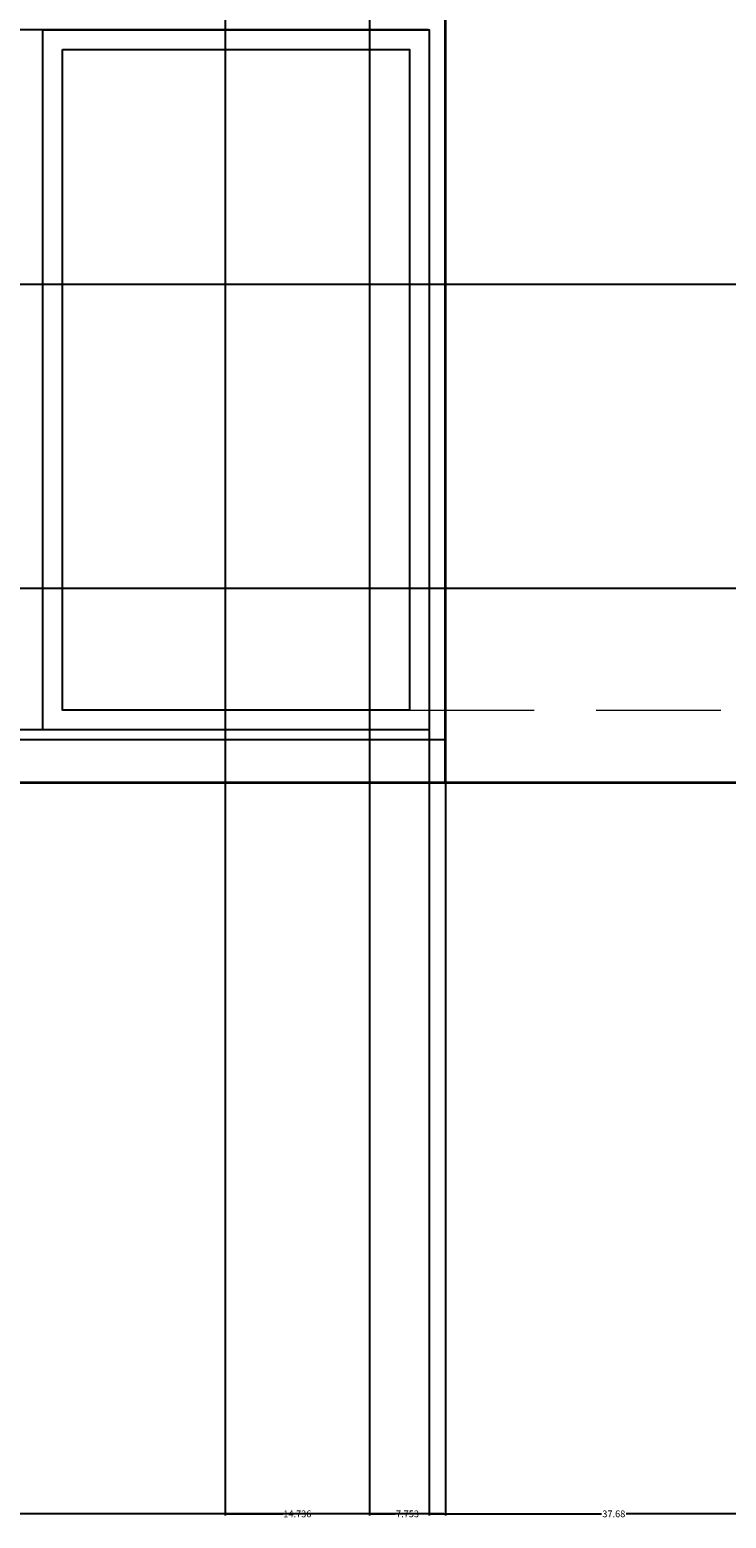
# Model space of a CAD drawing. Units: inches. Extents: x -145 to 510, y 5 to 386.
# Tile 16 of 25: x 275 to 346, y 5 to 157. Entities that reach past the tile are written whole.
import ezdxf

# ---------------------------------------------------------------- set-up
doc = ezdxf.new("R2010")
doc.units = ezdxf.units.IN
doc.header["$MEASUREMENT"] = 0
doc.linetypes.add('DASHED', pattern=[19.05, 12.7, -6.35])
for name, color, linetype, lineweight in [('A-ANNO-DIMS', 2, 'Continuous', 18), ('A-DOOR', 3, 'Continuous', 25), ('A-ELEV', 7, 'Continuous', 35), ('A-ELEV-HIDN', 8, 'DASHED', 18)]:
    doc.layers.add(name, color=color, linetype=linetype, lineweight=lineweight)
doc.styles.get("Standard").update_dxf_attribs({"font": 'arial.ttf'})
doc.dimstyles.get("Standard").update_dxf_attribs({"dimtxt": 0.6875, "dimasz": 0.18, "dimexe": 0.18, "dimexo": 0.0625, "dimgap": 0.09, "dimtad": 0, "dimtih": 1, "dimtoh": 1, "dimdec": 4, "dimzin": 0, "dimdsep": 46, "dimlunit": 4, "dimtxsty": 'Standard', "dimcen": 0.09, "dimadec": 0, "dimazin": 0, "dimtfac": 1, "dimtdec": 4, "dimtofl": 0, "dimtmove": 0, "dimatfit": 3, "dimfxl": 1, "dimtolj": 1, "dimtzin": 0, "dimarcsym": 0})

# ---------------------------------------------------------------- blocks, each defined once
blk = doc.blocks.new('*D10')
at = {"layer": 'A-ANNO-DIMS', "color": 0, "lineweight": -2, "transparency": 16777216}
for p, q in [((221.53, 85.2), (221.53, 5.19)), ((315.55, 85.2), (315.55, 5.19)), ((221.71, 5.37), (267.29, 5.37)), ((315.37, 5.37), (269.79, 5.37))]:
    blk.add_line(p, q, dxfattribs=at)
at = {"layer": 'A-ANNO-DIMS', "color": 0, "transparency": 16777216}
for points in [[(221.71, 5.4), (221.71, 5.34), (221.53, 5.37)], [(315.37, 5.4), (315.37, 5.34), (315.55, 5.37)]]:
    blk.add_solid(points, dxfattribs=at)
at = {"layer": 'Defpoints', "color": 0, "transparency": 16777216}
for p in [(221.53, 85.26), (315.55, 85.26), (315.55, 5.37)]:
    blk.add_point(p, dxfattribs=at)
at = {"layer": 'A-ANNO-DIMS', "color": 0, "transparency": 16777216, "insert": (268.54, 5.37), "char_height": 0.688, "attachment_point": 5}
blk.add_mtext('\\A1;94.03', dxfattribs=at)
blk = doc.blocks.new('*D11')
at = {"layer": 'A-ANNO-DIMS', "color": 0, "lineweight": -2, "transparency": 16777216}
for p, q in [((353.23, 115.19), (353.23, 5.19)), ((315.55, 85.2), (315.55, 5.19)), ((315.73, 5.37), (333.14, 5.37)), ((353.05, 5.37), (335.64, 5.37))]:
    blk.add_line(p, q, dxfattribs=at)
at = {"layer": 'A-ANNO-DIMS', "color": 0, "transparency": 16777216}
for points in [[(315.73, 5.4), (315.73, 5.34), (315.55, 5.37)], [(353.05, 5.4), (353.05, 5.34), (353.23, 5.37)]]:
    blk.add_solid(points, dxfattribs=at)
at = {"layer": 'Defpoints', "color": 0, "transparency": 16777216}
for p in [(353.23, 115.26), (315.55, 85.26), (353.23, 5.37)]:
    blk.add_point(p, dxfattribs=at)
at = {"layer": 'A-ANNO-DIMS', "color": 0, "transparency": 16777216, "insert": (334.39, 5.37), "char_height": 0.688, "attachment_point": 5}
blk.add_mtext('\\A1;37.68', dxfattribs=at)
blk = doc.blocks.new('*D19')
at = {"layer": 'A-ANNO-DIMS', "color": 0, "lineweight": -2, "transparency": 16777216}
for p, q in [((478.76, 355.89), (-144.05, 355.89)), ((-143.87, 355.71), (-143.87, 218.33)), ((-143.87, 80.07), (-143.87, 217.45)), ((-114.04, 79.89), (-144.05, 79.89))]:
    blk.add_line(p, q, dxfattribs=at)
at = {"layer": 'A-ANNO-DIMS', "color": 0, "transparency": 16777216}
for points in [[(-143.9, 355.71), (-143.84, 355.71), (-143.87, 355.89)], [(-143.9, 80.07), (-143.84, 80.07), (-143.87, 79.89)]]:
    blk.add_solid(points, dxfattribs=at)
at = {"layer": 'Defpoints', "color": 0, "transparency": 16777216}
for p in [(-143.87, 355.89), (478.83, 355.89), (-113.97, 79.89)]:
    blk.add_point(p, dxfattribs=at)
at = {"layer": 'A-ANNO-DIMS', "color": 0, "transparency": 16777216, "insert": (-143.87, 217.89), "char_height": 0.688, "attachment_point": 5}
blk.add_mtext('\\A1;276', dxfattribs=at)
blk = doc.blocks.new('*D47')
at = {"layer": 'A-ANNO-DIMS', "color": 0, "lineweight": -2, "transparency": 16777216}
for p, q in [((294.74, 279.78), (294.74, 5.19)), ((309.47, 271.83), (309.47, 5.19)), ((294.92, 5.37), (300.62, 5.37)), ((309.29, 5.37), (303.59, 5.37))]:
    blk.add_line(p, q, dxfattribs=at)
at = {"layer": 'A-ANNO-DIMS', "color": 0, "transparency": 16777216}
for points in [[(294.92, 5.4), (294.92, 5.34), (294.74, 5.37)], [(309.29, 5.4), (309.29, 5.34), (309.47, 5.37)]]:
    blk.add_solid(points, dxfattribs=at)
at = {"layer": 'Defpoints', "color": 0, "transparency": 16777216}
for p in [(294.74, 279.84), (309.47, 271.89), (309.47, 5.37)]:
    blk.add_point(p, dxfattribs=at)
at = {"layer": 'A-ANNO-DIMS', "color": 0, "transparency": 16777216, "insert": (302.11, 5.37), "char_height": 0.688, "attachment_point": 5}
blk.add_mtext('\\A1;14.736', dxfattribs=at)
blk = doc.blocks.new('*D48')
at = {"layer": 'A-ANNO-DIMS', "color": 0, "lineweight": -2, "transparency": 16777216}
for p, q in [((309.47, 223.83), (309.47, 5.19)), ((317.23, 223.83), (317.23, 5.19)), ((309.65, 5.37), (312.1, 5.37)), ((317.05, 5.37), (314.6, 5.37))]:
    blk.add_line(p, q, dxfattribs=at)
at = {"layer": 'A-ANNO-DIMS', "color": 0, "transparency": 16777216}
for points in [[(309.65, 5.4), (309.65, 5.34), (309.47, 5.37)], [(317.05, 5.4), (317.05, 5.34), (317.23, 5.37)]]:
    blk.add_solid(points, dxfattribs=at)
at = {"layer": 'Defpoints', "color": 0, "transparency": 16777216}
for p in [(309.47, 223.89), (317.23, 223.89), (317.23, 5.37)]:
    blk.add_point(p, dxfattribs=at)
at = {"layer": 'A-ANNO-DIMS', "color": 0, "transparency": 16777216, "insert": (313.35, 5.37), "char_height": 0.688, "attachment_point": 5}
blk.add_mtext('\\A1;7.753', dxfattribs=at)
blk = doc.blocks.new('*D54')
at = {"layer": 'A-ANNO-DIMS', "color": 0, "lineweight": -2, "transparency": 16777216}
for p, q in [((315.49, 156.61), (-144.05, 156.61)), ((-143.87, 156.43), (-143.87, 121.38)), ((-143.87, 85.44), (-143.87, 120.5)), ((315.49, 85.26), (-144.05, 85.26))]:
    blk.add_line(p, q, dxfattribs=at)
at = {"layer": 'A-ANNO-DIMS', "color": 0, "transparency": 16777216}
for points in [[(-143.9, 156.43), (-143.84, 156.43), (-143.87, 156.61)], [(-143.9, 85.44), (-143.84, 85.44), (-143.87, 85.26)]]:
    blk.add_solid(points, dxfattribs=at)
at = {"layer": 'Defpoints', "color": 0, "transparency": 16777216}
for p in [(-143.87, 156.61), (315.55, 156.61), (315.55, 85.26)]:
    blk.add_point(p, dxfattribs=at)
at = {"layer": 'A-ANNO-DIMS', "color": 0, "transparency": 16777216, "insert": (-143.87, 120.94), "char_height": 0.688, "attachment_point": 5}
blk.add_mtext('\\A1;71.35', dxfattribs=at)
blk = doc.blocks.new('*D58')
at = {"layer": 'A-ANNO-DIMS', "color": 0, "lineweight": -2, "transparency": 16777216}
for p, q in [((265.82, 130.67), (508.91, 130.67)), ((508.73, 130.49), (508.73, 115.63)), ((508.73, 99.89), (508.73, 114.75)), ((265.82, 99.71), (508.91, 99.71))]:
    blk.add_line(p, q, dxfattribs=at)
at = {"layer": 'A-ANNO-DIMS', "color": 0, "transparency": 16777216}
for points in [[(508.7, 130.49), (508.76, 130.49), (508.73, 130.67)], [(508.7, 99.89), (508.76, 99.89), (508.73, 99.71)]]:
    blk.add_solid(points, dxfattribs=at)
at = {"layer": 'Defpoints', "color": 0, "transparency": 16777216}
for p in [(265.76, 130.67), (508.73, 130.67), (265.76, 99.71)]:
    blk.add_point(p, dxfattribs=at)
at = {"layer": 'A-ANNO-DIMS', "color": 0, "transparency": 16777216, "insert": (508.73, 115.19), "char_height": 0.688, "attachment_point": 5}
blk.add_mtext('\\A1;30.96', dxfattribs=at)

msp = doc.modelspace()

# ---------------------------------------------------------------- linework, layer by layer
at = {"layer": 'A-DOOR'}
for p, q in [((271.4905, 84.2785), (278.1416, 84.2785)), ((278.1416, 84.2785), (313.5545, 84.2785)), ((313.5545, 84.2785), (317.2273, 84.2785))]:
    msp.add_line(p, q, dxfattribs=at)
for points in [[(276.1416, 156.6093), (315.5545, 156.6093), (315.5545, 85.2638), (276.1416, 85.2638)], [(278.1416, 154.6093), (313.5545, 154.6093), (313.5545, 87.2638), (278.1416, 87.2638)]]:
    msp.add_lwpolyline(points, close=True, dxfattribs=at)
at = {"layer": 'A-ELEV'}
for p, q in [((317.2273, 79.8905), (317.2273, 223.8905)), ((54.0014, 79.8905), (392.4492, 79.8905))]:
    msp.add_line(p, q, dxfattribs=at)
at = {"layer": 'A-ELEV-HIDN'}
msp.add_line((313.5545, 87.2638), (474.4893, 87.2638), dxfattribs=at)

# ---------------------------------------------------------------- dimensions: what is measured, and where the dimension line sits
at = {"layer": 'A-ANNO-DIMS'}
for base, p1, p2, override, picture, middle in [((-143.8737, 355.8905), (-113.9737, 79.8905), (478.8263, 355.8905), {"dimdec": 0, "dimlfac": 1, "dimrnd": 0, "dimzin": 0, "dimdsep": 46, "dimlunit": 2}, '*D19', (-143.8737, 217.8905)), ((-143.8737, 156.6093), (315.5545, 85.2638), (315.5545, 156.6093), {"dimdec": 2, "dimlfac": 1, "dimrnd": 0, "dimzin": 0, "dimdsep": 46, "dimlunit": 2}, '*D54', (-143.8737, 120.9365)), ((508.7263, 130.6707), (265.7612, 99.7118), (265.7612, 130.6707), {"dimdec": 2, "dimlfac": 1, "dimrnd": 0, "dimzin": 0, "dimdsep": 46, "dimlunit": 2}, '*D58', (508.7263, 115.1912))]:
    dim = msp.add_linear_dim(base=base, p1=p1, p2=p2, angle=90, dimstyle='Standard', override=override, dxfattribs=at)
    dim.commit()
    dim.dimension.update_dxf_attribs({"geometry": picture, "text_midpoint": middle})
for base, p1, p2, override, picture, middle in [((309.4739, 5.3738), (294.738, 279.8443), (309.4739, 271.8905), {"dimdec": 3, "dimlfac": 1, "dimrnd": 0, "dimzin": 0, "dimdsep": 46, "dimlunit": 2}, '*D47', (302.106, 5.3738)), ((317.2273, 5.3738), (309.4739, 223.8905), (317.2273, 223.8905), {"dimdec": 3, "dimlfac": 1, "dimrnd": 0, "dimzin": 0, "dimdsep": 46, "dimlunit": 2}, '*D48', (313.3506, 5.3738)), ((353.234, 5.3738), (315.5545, 85.2638), (353.234, 115.2574), {"dimdec": 2, "dimlfac": 1, "dimrnd": 0, "dimzin": 0, "dimdsep": 46, "dimlunit": 2}, '*D11', (334.3942, 5.3738)), ((315.5545, 5.3738), (221.5292, 85.2638), (315.5545, 85.2638), {"dimdec": 2, "dimlfac": 1, "dimrnd": 0, "dimzin": 0, "dimdsep": 46, "dimlunit": 2}, '*D10', (268.5418, 5.3738))]:
    dim = msp.add_linear_dim(base=base, p1=p1, p2=p2, dimstyle='Standard', override=override, dxfattribs=at)
    dim.commit()
    dim.dimension.update_dxf_attribs({"geometry": picture, "text_midpoint": middle})

doc.saveas('drawing.dxf')
